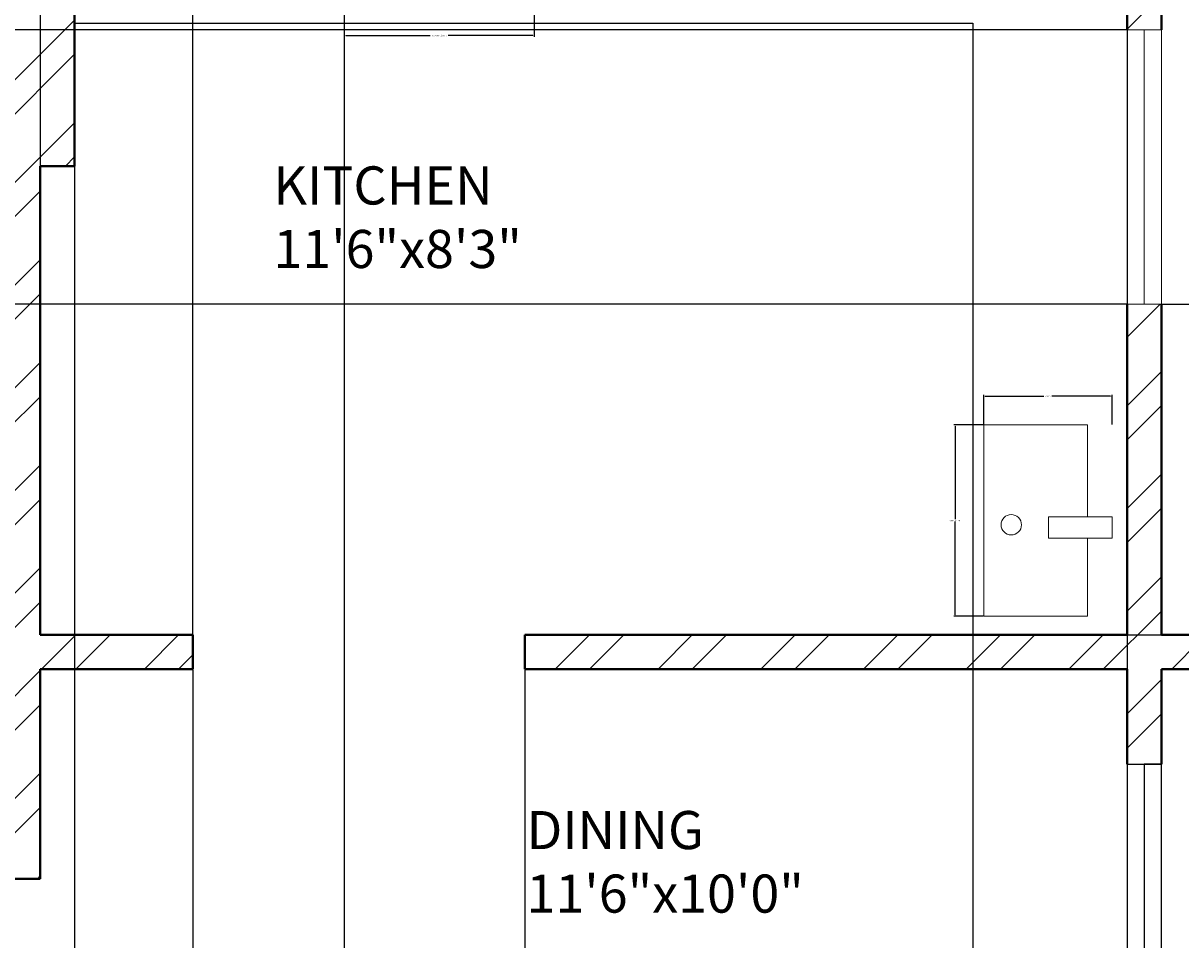
# Model space of a CAD drawing. Units: inches. Extents: x 1601 to 2297, y 1496 to 2631.
# Tile 27 of 57: x 2033 to 2185, y 1946 to 2067. Entities that reach past the tile are written whole.
import ezdxf

# ---------------------------------------------------------------- set-up
doc = ezdxf.new("R2010")
doc.units = ezdxf.units.IN
for name, color, linetype, lineweight in [('A-ANNO-DIMS', 2, 'Continuous', 18), ('A-AREA-IDEN', 7, 'Continuous', 18), ('A-DOOR', 21, 'Continuous', 25), ('A-FLOR-CASE', 8, 'Continuous', 25), ('A-FLOR-FIXT', 9, 'Continuous', 20), ('A-GLAZ', 161, 'Continuous', 20), ('A-WALL', 7, 'Continuous', 40), ('A-WALL-PATT', 215, 'Continuous', 13)]:
    doc.layers.add(name, color=color, linetype=linetype, lineweight=lineweight)
doc.styles.get("Standard").update_dxf_attribs({"font": 'arial.ttf'})
doc.dimstyles.get("Standard").update_dxf_attribs({"dimtxt": 0.18, "dimasz": 0.18, "dimexe": 0.18, "dimexo": 0.0625, "dimgap": 0.09, "dimtad": 0, "dimtih": 1, "dimtoh": 1, "dimdec": 4, "dimzin": 0, "dimdsep": 46, "dimtxsty": 'Standard', "dimcen": 0.09, "dimadec": 0, "dimazin": 0, "dimtfac": 1, "dimtdec": 4, "dimtofl": 0, "dimtmove": 0, "dimatfit": 3, "dimfxl": 1, "dimtolj": 1, "dimtzin": 0, "dimarcsym": 0})

# ---------------------------------------------------------------- blocks, each defined once
blk = doc.blocks.new('SINK-KITCHEN')
blk.add_lwpolyline([(13.62, 10.25), (13.62, 0), (0, 0), (0, 25.08), (13.62, 25.08), (13.62, 13.01)])
blk.add_lwpolyline([(8.47, 13.01), (16.82, 13.01), (16.82, 10.25), (8.47, 10.25)], close=True)
blk.add_circle((3.61, 11.99), 1.34)
blk = doc.blocks.new('*D18')
at = {"layer": 'A-ANNO-DIMS', "color": 0, "lineweight": -2, "transparency": 16777216}
for p, q in [((2075.4, 2068.63), (2075.4, 2064.77)), ((2100.29, 2068.63), (2100.29, 2064.77)), ((2075.58, 2064.95), (2086.65, 2064.95)), ((2100.11, 2064.95), (2089.03, 2064.95))]:
    blk.add_line(p, q, dxfattribs=at)
at = {"layer": 'A-ANNO-DIMS', "color": 0, "transparency": 16777216}
for points in [[(2075.58, 2064.98), (2075.58, 2064.92), (2075.4, 2064.95)], [(2100.11, 2064.98), (2100.11, 2064.92), (2100.29, 2064.95)]]:
    blk.add_solid(points, dxfattribs=at)
at = {"layer": 'Defpoints', "color": 0, "transparency": 16777216}
for p in [(2075.4, 2068.69), (2100.29, 2068.69), (2100.29, 2064.95)]:
    blk.add_point(p, dxfattribs=at)
at = {"layer": 'A-ANNO-DIMS', "color": 0, "transparency": 16777216, "insert": (2087.84, 2064.95), "char_height": 0.18, "attachment_point": 5}
blk.add_mtext('\\A1;COOKTOP 25 TYP.', dxfattribs=at)
blk = doc.blocks.new('*D20')
at = {"layer": 'A-ANNO-DIMS', "color": 0, "lineweight": -2, "transparency": 16777216}
for p, q in [((2159.18, 2013.87), (2155.3, 2013.87)), ((2155.48, 2013.69), (2155.48, 2001.51)), ((2155.48, 1988.97), (2155.48, 2001.14)), ((2159.18, 1988.79), (2155.3, 1988.79))]:
    blk.add_line(p, q, dxfattribs=at)
at = {"layer": 'A-ANNO-DIMS', "color": 0, "transparency": 16777216}
for points in [[(2155.45, 2013.69), (2155.51, 2013.69), (2155.48, 2013.87)], [(2155.45, 1988.97), (2155.51, 1988.97), (2155.48, 1988.79)]]:
    blk.add_solid(points, dxfattribs=at)
at = {"layer": 'Defpoints', "color": 0, "transparency": 16777216}
for p in [(2155.48, 2013.87), (2159.24, 2013.87), (2159.24, 1988.79)]:
    blk.add_point(p, dxfattribs=at)
at = {"layer": 'A-ANNO-DIMS', "color": 0, "transparency": 16777216, "insert": (2155.48, 2001.33), "char_height": 0.18, "attachment_point": 5}
blk.add_mtext('\\A1;SINK 25 TYP.', dxfattribs=at)
blk = doc.blocks.new('*D21')
at = {"layer": 'A-ANNO-DIMS', "color": 0, "lineweight": -2, "transparency": 16777216}
for p, q in [((2159.24, 2013.93), (2159.24, 2017.81)), ((2159.42, 2017.63), (2167.13, 2017.63)), ((2175.88, 2017.63), (2168.17, 2017.63)), ((2176.06, 2013.93), (2176.06, 2017.81))]:
    blk.add_line(p, q, dxfattribs=at)
at = {"layer": 'A-ANNO-DIMS', "color": 0, "transparency": 16777216}
for points in [[(2159.42, 2017.66), (2159.42, 2017.6), (2159.24, 2017.63)], [(2175.88, 2017.66), (2175.88, 2017.6), (2176.06, 2017.63)]]:
    blk.add_solid(points, dxfattribs=at)
at = {"layer": 'Defpoints', "color": 0, "transparency": 16777216}
for p in [(2176.06, 2017.63), (2159.24, 2013.87), (2176.06, 2013.87)]:
    blk.add_point(p, dxfattribs=at)
at = {"layer": 'A-ANNO-DIMS', "color": 0, "transparency": 16777216, "insert": (2167.65, 2017.63), "char_height": 0.18, "attachment_point": 5}
blk.add_mtext('\\A1;17 TYP.', dxfattribs=at)
blk = doc.blocks.new('*D38')
at = {"layer": 'A-ANNO-DIMS', "color": 0, "lineweight": -2, "transparency": 16777216}
for p, q in [((2178.04, 2085.26), (2178.04, 1513.75)), ((2157.8, 2066.51), (2157.8, 1513.75)), ((2157.98, 1513.93), (2167.52, 1513.93)), ((2177.86, 1513.93), (2168.31, 1513.93))]:
    blk.add_line(p, q, dxfattribs=at)
at = {"layer": 'A-ANNO-DIMS', "color": 0, "transparency": 16777216}
for points in [[(2157.98, 1513.96), (2157.98, 1513.9), (2157.8, 1513.93)], [(2177.86, 1513.96), (2177.86, 1513.9), (2178.04, 1513.93)]]:
    blk.add_solid(points, dxfattribs=at)
at = {"layer": 'Defpoints', "color": 0, "transparency": 16777216}
for p in [(2178.04, 2085.33), (2157.8, 2066.58), (2178.04, 1513.93)]:
    blk.add_point(p, dxfattribs=at)
at = {"layer": 'A-ANNO-DIMS', "color": 0, "transparency": 16777216, "insert": (2167.92, 1513.93), "char_height": 0.18, "attachment_point": 5}
blk.add_mtext('\\A1;20.24', dxfattribs=at)
blk = doc.blocks.new('*D39')
at = {"layer": 'A-ANNO-DIMS', "color": 0, "lineweight": -2, "transparency": 16777216}
for p, q in [((2055.55, 1981.76), (2055.55, 1513.75)), ((2099.05, 1981.76), (2099.05, 1513.75)), ((2055.73, 1513.93), (2076.97, 1513.93)), ((2098.87, 1513.93), (2077.63, 1513.93))]:
    blk.add_line(p, q, dxfattribs=at)
at = {"layer": 'A-ANNO-DIMS', "color": 0, "transparency": 16777216}
for points in [[(2055.73, 1513.96), (2055.73, 1513.9), (2055.55, 1513.93)], [(2098.87, 1513.96), (2098.87, 1513.9), (2099.05, 1513.93)]]:
    blk.add_solid(points, dxfattribs=at)
at = {"layer": 'Defpoints', "color": 0, "transparency": 16777216}
for p in [(2055.55, 1981.83), (2099.05, 1981.83), (2099.05, 1513.93)]:
    blk.add_point(p, dxfattribs=at)
at = {"layer": 'A-ANNO-DIMS', "color": 0, "transparency": 16777216, "insert": (2077.3, 1513.93), "char_height": 0.18, "attachment_point": 5}
blk.add_mtext('\\A1;43.5', dxfattribs=at)
blk = doc.blocks.new('*D40')
at = {"layer": 'A-ANNO-DIMS', "color": 0, "lineweight": -2, "transparency": 16777216}
for p, q in [((2035.54, 1986.39), (2035.54, 2581.06)), ((2035.72, 2580.88), (2045.08, 2580.88)), ((2055.37, 2580.88), (2046.01, 2580.88)), ((2055.55, 1986.39), (2055.55, 2581.06))]:
    blk.add_line(p, q, dxfattribs=at)
at = {"layer": 'A-ANNO-DIMS', "color": 0, "transparency": 16777216}
for points in [[(2035.72, 2580.91), (2035.72, 2580.85), (2035.54, 2580.88)], [(2055.37, 2580.91), (2055.37, 2580.85), (2055.55, 2580.88)]]:
    blk.add_solid(points, dxfattribs=at)
at = {"layer": 'Defpoints', "color": 0, "transparency": 16777216}
for p in [(2055.55, 2580.88), (2035.54, 1986.33), (2055.55, 1986.33)]:
    blk.add_point(p, dxfattribs=at)
at = {"layer": 'A-ANNO-DIMS', "color": 0, "transparency": 16777216, "insert": (2045.54, 2580.88), "char_height": 0.18, "attachment_point": 5}
blk.add_mtext('\\A1;20.014', dxfattribs=at)
blk = doc.blocks.new('*D41')
at = {"layer": 'A-ANNO-DIMS', "color": 0, "lineweight": -2, "transparency": 16777216}
for p, q in [((2075.4, 2070.14), (2075.4, 1513.75)), ((2040.04, 2066.51), (2040.04, 1513.75)), ((2040.22, 1513.93), (2057.32, 1513.93)), ((2075.22, 1513.93), (2058.11, 1513.93))]:
    blk.add_line(p, q, dxfattribs=at)
at = {"layer": 'A-ANNO-DIMS', "color": 0, "transparency": 16777216}
for points in [[(2040.22, 1513.96), (2040.22, 1513.9), (2040.04, 1513.93)], [(2075.22, 1513.96), (2075.22, 1513.9), (2075.4, 1513.93)]]:
    blk.add_solid(points, dxfattribs=at)
at = {"layer": 'Defpoints', "color": 0, "transparency": 16777216}
for p in [(2075.4, 2070.2), (2040.04, 2066.58), (2075.4, 1513.93)]:
    blk.add_point(p, dxfattribs=at)
at = {"layer": 'A-ANNO-DIMS', "color": 0, "transparency": 16777216, "insert": (2057.72, 1513.93), "char_height": 0.18, "attachment_point": 5}
blk.add_mtext('\\A1;35.36', dxfattribs=at)
blk = doc.blocks.new('*D42')
at = {"layer": 'A-ANNO-DIMS', "color": 0, "lineweight": -2, "transparency": 16777216}
for p, q in [((2177.97, 2065.7), (1637.31, 2065.7)), ((1637.49, 2065.52), (1637.49, 2047.88)), ((1637.49, 2029.88), (1637.49, 2047.51)), ((2177.97, 2029.7), (1637.31, 2029.7))]:
    blk.add_line(p, q, dxfattribs=at)
at = {"layer": 'A-ANNO-DIMS', "color": 0, "transparency": 16777216}
for points in [[(1637.46, 2065.52), (1637.52, 2065.52), (1637.49, 2065.7)], [(1637.46, 2029.88), (1637.52, 2029.88), (1637.49, 2029.7)]]:
    blk.add_solid(points, dxfattribs=at)
at = {"layer": 'Defpoints', "color": 0, "transparency": 16777216}
for p in [(1637.49, 2065.7), (2178.04, 2065.7), (2178.04, 2029.7)]:
    blk.add_point(p, dxfattribs=at)
at = {"layer": 'A-ANNO-DIMS', "color": 0, "transparency": 16777216, "insert": (1637.49, 2047.7), "char_height": 0.18, "attachment_point": 5}
blk.add_mtext('\\A1;36', dxfattribs=at)
blk = doc.blocks.new('*D43')
at = {"layer": 'A-ANNO-DIMS', "color": 0, "lineweight": -2, "transparency": 16777216}
for p, q in [((2182.6, 2029.7), (2279.27, 2029.7)), ((2279.09, 2029.52), (2279.09, 2008.19)), ((2279.09, 1986.51), (2279.09, 2007.83)), ((2178.1, 1986.33), (2279.27, 1986.33))]:
    blk.add_line(p, q, dxfattribs=at)
at = {"layer": 'A-ANNO-DIMS', "color": 0, "transparency": 16777216}
for points in [[(2279.06, 2029.52), (2279.12, 2029.52), (2279.09, 2029.7)], [(2279.06, 1986.51), (2279.12, 1986.51), (2279.09, 1986.33)]]:
    blk.add_solid(points, dxfattribs=at)
at = {"layer": 'Defpoints', "color": 0, "transparency": 16777216}
for p in [(2182.54, 2029.7), (2178.04, 1986.33), (2279.09, 1986.33)]:
    blk.add_point(p, dxfattribs=at)
at = {"layer": 'A-ANNO-DIMS', "color": 0, "transparency": 16777216, "insert": (2279.09, 2008.01), "char_height": 0.18, "attachment_point": 5}
blk.add_mtext('\\A1;43.37', dxfattribs=at)

msp = doc.modelspace()

# ---------------------------------------------------------------- hatches: boundary and pattern name
at = {"layer": 'A-WALL-PATT'}
h = msp.add_hatch(dxfattribs=at)
h.set_pattern_fill('ANSI32', color=256)
h.paths.add_polyline_path([(1842.0336, 2528.0767), (1842.0336, 2532.3254), (1686.0373, 2532.3254), (1686.0373, 2492.9493), (1695.0373, 2492.9493), (1695.0373, 2523.3254), (1827.0373, 2523.3254), (1827.0373, 2416.8254), (1834.6225, 2416.8254), (1834.6225, 2419.0754), (1834.6225, 2421.3254), (1831.5373, 2421.3254), (1831.5373, 2523.3254), (1842.0336, 2523.3254)])
h.paths.add_polyline_path([(1695.0373, 2432.9493), (1686.0373, 2432.9493), (1686.0373, 2325.989), (1695.0373, 2325.989), (1695.0373, 2347.8254), (1827.0373, 2347.8254), (1827.0373, 2287.8254), (1823.2991, 2287.8254), (1823.2991, 2283.3254), (1847.9422, 2283.3254), (1847.9422, 2285.5754), (1847.9422, 2287.8254), (1831.5373, 2287.8254), (1831.5373, 2347.8254), (1846.9946, 2347.8254), (1846.9946, 2350.0754), (1846.9946, 2352.3254), (1695.0373, 2352.3254)])
h.paths.add_polyline_path([(1807.1169, 1573.5395), (2055.0405, 1573.5395), (2055.0405, 1610.6322), (1807.1169, 1610.6322)], flags=9)
h.paths.add_polyline_path([(1841.1631, 1712.7967), (1870.3957, 1712.7967), (1870.3957, 1731.454), (1841.1631, 1731.454)], flags=9)
h.paths.add_polyline_path([(2144.3862, 1772.185), (2191.0233, 1772.185), (2191.0233, 1790.8423), (2144.3862, 1790.8423)], flags=9)
h.paths.add_polyline_path([(2143.0128, 1827.3312), (2177.9958, 1827.3312), (2177.9958, 1845.9886), (2143.0128, 1845.9886)], flags=9)
h.paths.add_polyline_path([(2041.2439, 1833.5691), (2070.8516, 1833.5691), (2070.8516, 1852.2264), (2041.2439, 1852.2264)], flags=9)
h.paths.add_polyline_path([(2097.2791, 1947.0598), (2134.2061, 1947.0598), (2134.2061, 1965.7171), (2097.2791, 1965.7171)], flags=9)
h.paths.add_polyline_path([(2214.995, 1904.3124), (2214.995, 1942.2899), (2196.3376, 1942.2899), (2196.3376, 1904.3124)], flags=9)
h.paths.add_polyline_path([(2186.6284, 2043.8031), (2219.7935, 2043.8031), (2219.7935, 2062.4605), (2186.6284, 2062.4605)], flags=9)
h.paths.add_polyline_path([(2064.0877, 2031.616), (2097.4949, 2031.616), (2097.4949, 2050.2734), (2064.0877, 2050.2734)], flags=9)
h.paths.add_polyline_path([(1973.1349, 1986.0688), (2008.4009, 1986.0688), (2008.4009, 2004.7261), (1973.1349, 2004.7261)], flags=9)
h.paths.add_polyline_path([(1976.3676, 2106.9635), (2005.7469, 2106.9635), (2005.7469, 2125.6209), (1976.3676, 2125.6209)], flags=9)
h.paths.add_polyline_path([(1991.7852, 2180.4863), (2027.0513, 2180.4863), (2027.0513, 2199.1437), (1991.7852, 2199.1437)], flags=9)
h.paths.add_polyline_path([(2106.1801, 2187.9359), (2152.2101, 2187.9359), (2152.2101, 2206.5932), (2106.1801, 2206.5932)], flags=9)
h.paths.add_polyline_path([(2148.6686, 2262.2542), (2182.318, 2262.2542), (2182.318, 2280.9115), (2148.6686, 2280.9115)], flags=9)
h.paths.add_polyline_path([(2041.6327, 2252.8147), (2071.2405, 2252.8147), (2071.2405, 2271.4721), (2041.6327, 2271.4721)], flags=9)
h.paths.add_polyline_path([(2063.9734, 2375.4265), (2100.9004, 2375.4265), (2100.9004, 2394.0839), (2063.9734, 2394.0839)], flags=9)
h.paths.add_polyline_path([(2216.4955, 2330.9748), (2216.4955, 2370.2654), (2197.8381, 2370.2654), (2197.8381, 2330.9748)], flags=9)
h.paths.add_polyline_path([(2179.1416, 2485.8687), (2212.3067, 2485.8687), (2212.3067, 2504.5261), (2179.1416, 2504.5261)], flags=9)
h.paths.add_polyline_path([(2078.7442, 2471.1516), (2112.1514, 2471.1516), (2112.1514, 2489.809), (2078.7442, 2489.809)], flags=9)
h.paths.add_polyline_path([(1915.9631, 2329.4668), (1952.8902, 2329.4668), (1952.8902, 2348.1241), (1915.9631, 2348.1241)], flags=9)
h.paths.add_polyline_path([(1904.3189, 2499.6709), (1940.4512, 2499.6709), (1940.4512, 2518.3282), (1904.3189, 2518.3282)], flags=9)
h.paths.add_polyline_path([(1892.3665, 2100.4595), (1925.6374, 2100.4595), (1925.6374, 2119.1169), (1892.3665, 2119.1169)], flags=9)
h.paths.add_polyline_path([(1909.2984, 1805.9631), (1946.2254, 1805.9631), (1946.2254, 1824.6205), (1909.2984, 1824.6205)], flags=9)
h.paths.add_polyline_path([(1934.6056, 1658.616), (1970.738, 1658.616), (1970.738, 1677.2733), (1934.6056, 1677.2733)], flags=9)
h.paths.add_polyline_path([(1711.2052, 1789.8902), (1750.0456, 1789.8902), (1750.0456, 1808.5476), (1711.2052, 1808.5476)], flags=9)
h.paths.add_polyline_path([(1742.7874, 1854.6743), (1771.9449, 1854.6743), (1771.9449, 1873.3317), (1742.7874, 1873.3317)], flags=9)
h.paths.add_polyline_path([(1807.3592, 1997.7912), (1850.1116, 1997.7912), (1850.1116, 2016.4486), (1807.3592, 2016.4486)], flags=9)
h.paths.add_polyline_path([(1717.4579, 2237.7844), (1760.2103, 2237.7844), (1760.2103, 2256.4417), (1717.4579, 2256.4417)], flags=9)
h.paths.add_polyline_path([(1780.9285, 2324.0623), (1810.086, 2324.0623), (1810.086, 2342.7197), (1780.9285, 2342.7197)], flags=25)
h.paths.add_polyline_path([(1837.696, 2449.2024), (1866.9286, 2449.2024), (1866.9286, 2467.8598), (1837.696, 2467.8598)], flags=9)
h.paths.add_polyline_path([(1712.7752, 2484.9404), (1751.6156, 2484.9404), (1751.6156, 2503.5977), (1712.7752, 2503.5977)], flags=25)
h = msp.add_hatch(dxfattribs=at)
h.set_pattern_fill('ANSI32', color=256)
h.paths.add_polyline_path([(1973.9371, 2211.3254), (1893.0373, 2211.3254), (1893.0373, 2287.8254), (1884.6167, 2287.8254), (1884.6167, 2285.5754), (1884.6167, 2283.3254), (1888.5373, 2283.3254), (1888.5373, 2145.3254), (1695.0373, 2145.3254), (1695.0373, 2173.8724), (1690.5373, 2173.8724), (1686.0373, 2173.8724), (1686.0373, 2136.3254), (1722.5687, 2136.3254), (1722.5687, 2117.4352), (1731.5687, 2117.4352), (1731.5687, 2136.3254), (1893.0373, 2136.3254), (1893.0373, 2202.3254), (1959.0373, 2202.3254), (1959.0373, 2182.1303), (1968.0373, 2182.1303), (1968.0373, 2202.3254), (1973.9371, 2202.3254)])
h.paths.add_polyline_path([(2094.0373, 2274.6364), (2096.4294, 2274.6364), (2096.4294, 2276.8864), (2096.4294, 2279.1364), (2094.0373, 2279.1364), (2094.0373, 2290.8254), (2094.0373, 2295.3254), (2089.5373, 2295.3254), (2089.5373, 2230.8254), (2035.5373, 2230.8254), (2035.5373, 2299.8254), (2031.0373, 2299.8254), (2031.0373, 2211.3254), (2023.0065, 2211.3254), (2023.0065, 2202.3254), (2031.0373, 2202.3254), (2031.0373, 2140.8254), (1968.0373, 2140.8254), (1968.0373, 2145.9106), (1963.5373, 2145.9106), (1959.0373, 2145.9106), (1959.0373, 2116.839), (1963.5373, 2116.839), (1968.0373, 2116.839), (1968.0373, 2131.8254), (2031.0373, 2131.8254), (2031.0373, 2094.3254), (2031.0373, 2085.3254), (2031.0373, 2056.8254), (1968.0373, 2056.8254), (1968.0373, 2070.4947), (1963.5373, 2070.4947), (1959.0373, 2070.4947), (1959.0373, 2040.3029), (1968.0373, 2040.3029), (1968.0373, 2047.8254), (2031.0373, 2047.8254), (2031.0373, 1983.3254), (2031.0373, 1978.8254), (2021.1979, 1978.8254), (2021.1979, 1974.3254), (2031.0373, 1974.3254), (2031.0373, 1954.3528), (2035.5373, 1954.3528), (2035.5373, 1974.3254), (2035.5373, 1981.8254), (2055.5513, 1981.8254), (2055.5513, 1986.3254), (2035.5373, 1986.3254), (2035.5373, 2047.8254), (2040.0373, 2047.8254), (2040.0373, 2085.3254), (2040.0373, 2094.3254), (2040.0373, 2140.8254), (2035.5373, 2140.8254), (2035.5373, 2226.3254), (2089.5373, 2226.3254), (2094.0373, 2226.3254)])
h.paths.add_polyline_path([(2226.0373, 2230.8254), (2134.5373, 2230.8254), (2134.5373, 2233.5437), (2130.0373, 2233.5437), (2130.0373, 2226.3254), (2134.5373, 2226.3254), (2226.0373, 2226.3254)])
h.paths.add_polyline_path([(1807.1169, 1573.5395), (2055.0405, 1573.5395), (2055.0405, 1610.6322), (1807.1169, 1610.6322)], flags=9)
h.paths.add_polyline_path([(1841.1631, 1712.7967), (1870.3957, 1712.7967), (1870.3957, 1731.454), (1841.1631, 1731.454)], flags=9)
h.paths.add_polyline_path([(2144.3862, 1772.185), (2191.0233, 1772.185), (2191.0233, 1790.8423), (2144.3862, 1790.8423)], flags=9)
h.paths.add_polyline_path([(2143.0128, 1827.3312), (2177.9958, 1827.3312), (2177.9958, 1845.9886), (2143.0128, 1845.9886)], flags=9)
h.paths.add_polyline_path([(2041.2439, 1833.5691), (2070.8516, 1833.5691), (2070.8516, 1852.2264), (2041.2439, 1852.2264)], flags=9)
h.paths.add_polyline_path([(2097.2791, 1947.0598), (2134.2061, 1947.0598), (2134.2061, 1965.7171), (2097.2791, 1965.7171)], flags=9)
h.paths.add_polyline_path([(2214.995, 1904.3124), (2214.995, 1942.2899), (2196.3376, 1942.2899), (2196.3376, 1904.3124)], flags=9)
h.paths.add_polyline_path([(2186.6284, 2043.8031), (2219.7935, 2043.8031), (2219.7935, 2062.4605), (2186.6284, 2062.4605)], flags=9)
h.paths.add_polyline_path([(2064.0877, 2031.616), (2097.4949, 2031.616), (2097.4949, 2050.2734), (2064.0877, 2050.2734)], flags=9)
h.paths.add_polyline_path([(1973.1349, 1986.0688), (2008.4009, 1986.0688), (2008.4009, 2004.7261), (1973.1349, 2004.7261)], flags=25)
h.paths.add_polyline_path([(1976.3676, 2106.9635), (2005.7469, 2106.9635), (2005.7469, 2125.6209), (1976.3676, 2125.6209)], flags=25)
h.paths.add_polyline_path([(1991.7852, 2180.4863), (2027.0513, 2180.4863), (2027.0513, 2199.1437), (1991.7852, 2199.1437)], flags=25)
h.paths.add_polyline_path([(2106.1801, 2187.9359), (2152.2101, 2187.9359), (2152.2101, 2206.5932), (2106.1801, 2206.5932)], flags=9)
h.paths.add_polyline_path([(2148.6686, 2262.2542), (2182.318, 2262.2542), (2182.318, 2280.9115), (2148.6686, 2280.9115)], flags=9)
h.paths.add_polyline_path([(2041.6327, 2252.8147), (2071.2405, 2252.8147), (2071.2405, 2271.4721), (2041.6327, 2271.4721)], flags=25)
h.paths.add_polyline_path([(2063.9734, 2375.4265), (2100.9004, 2375.4265), (2100.9004, 2394.0839), (2063.9734, 2394.0839)], flags=9)
h.paths.add_polyline_path([(2216.4955, 2330.9748), (2216.4955, 2370.2654), (2197.8381, 2370.2654), (2197.8381, 2330.9748)], flags=9)
h.paths.add_polyline_path([(2179.1416, 2485.8687), (2212.3067, 2485.8687), (2212.3067, 2504.5261), (2179.1416, 2504.5261)], flags=9)
h.paths.add_polyline_path([(2078.7442, 2471.1516), (2112.1514, 2471.1516), (2112.1514, 2489.809), (2078.7442, 2489.809)], flags=9)
h.paths.add_polyline_path([(1915.9631, 2329.4668), (1952.8902, 2329.4668), (1952.8902, 2348.1241), (1915.9631, 2348.1241)], flags=9)
h.paths.add_polyline_path([(1904.3189, 2499.6709), (1940.4512, 2499.6709), (1940.4512, 2518.3282), (1904.3189, 2518.3282)], flags=9)
h.paths.add_polyline_path([(1892.3665, 2100.4595), (1925.6374, 2100.4595), (1925.6374, 2119.1169), (1892.3665, 2119.1169)], flags=9)
h.paths.add_polyline_path([(1909.2984, 1805.9631), (1946.2254, 1805.9631), (1946.2254, 1824.6205), (1909.2984, 1824.6205)], flags=9)
h.paths.add_polyline_path([(1934.6056, 1658.616), (1970.738, 1658.616), (1970.738, 1677.2733), (1934.6056, 1677.2733)], flags=9)
h.paths.add_polyline_path([(1711.2052, 1789.8902), (1750.0456, 1789.8902), (1750.0456, 1808.5476), (1711.2052, 1808.5476)], flags=9)
h.paths.add_polyline_path([(1742.7874, 1854.6743), (1771.9449, 1854.6743), (1771.9449, 1873.3317), (1742.7874, 1873.3317)], flags=9)
h.paths.add_polyline_path([(1807.3592, 1997.7912), (1850.1116, 1997.7912), (1850.1116, 2016.4486), (1807.3592, 2016.4486)], flags=9)
h.paths.add_polyline_path([(1717.4579, 2237.7844), (1760.2103, 2237.7844), (1760.2103, 2256.4417), (1717.4579, 2256.4417)], flags=25)
h.paths.add_polyline_path([(1780.9285, 2324.0623), (1810.086, 2324.0623), (1810.086, 2342.7197), (1780.9285, 2342.7197)], flags=9)
h.paths.add_polyline_path([(1837.696, 2449.2024), (1866.9286, 2449.2024), (1866.9286, 2467.8598), (1837.696, 2467.8598)], flags=9)
h.paths.add_polyline_path([(1712.7752, 2484.9404), (1751.6156, 2484.9404), (1751.6156, 2503.5977), (1712.7752, 2503.5977)], flags=9)
h = msp.add_hatch(dxfattribs=at)
h.set_pattern_fill('ANSI32', color=256)
h.paths.add_polyline_path([(2230.5373, 1861.8254), (2182.5373, 1861.8254), (2182.5373, 1885.3637), (2178.0373, 1885.3637), (2178.0373, 1861.8254), (2166.0373, 1861.8254), (2134.5373, 1861.8254), (2130.0373, 1861.8254), (2130.0373, 1841.4682), (2126.8833, 1841.4682), (2126.8833, 1836.9682), (2130.0373, 1836.9682), (2130.0373, 1822.7302), (2134.5373, 1822.7302), (2134.5373, 1857.3254), (2166.0373, 1857.3254), (2226.0373, 1857.3254), (2226.0373, 1846.1155), (2230.5373, 1846.1155)])
h.paths.add_polyline_path([(2226.0373, 1797.3254), (2134.5373, 1797.3254), (2134.5373, 1800.6636), (2132.2873, 1800.6636), (2130.0373, 1800.6636), (2130.0373, 1797.3254), (2130.0373, 1792.8254), (2167.7264, 1792.8254), (2226.0373, 1792.8254)])
h.paths.add_polyline_path([(2230.5373, 1822.1155), (2226.0373, 1822.1155), (2226.0373, 1760.8563), (2230.5373, 1760.8563)])
h.paths.add_polyline_path([(2230.5373, 1700.8563), (2226.0373, 1700.8563), (2226.0373, 1644.3254), (2140.2517, 1644.3254), (2140.2517, 1635.3254), (2230.5373, 1635.3254)])
h.paths.add_polyline_path([(2080.2517, 1639.8254), (2080.2517, 1644.3254), (2035.5373, 1644.3254), (2035.5373, 1792.8254), (2094.0373, 1792.8254), (2094.0373, 1797.3254), (2094.0373, 1836.9682), (2097.1057, 1836.9682), (2097.1057, 1839.2182), (2097.1057, 1841.4682), (2094.0373, 1841.4682), (2094.0373, 1862.2276), (2089.5373, 1862.2276), (2089.5373, 1797.3254), (2035.5373, 1797.3254), (2035.5373, 1857.3254), (2035.5373, 1885.0916), (2031.0373, 1885.0916), (2031.0373, 1710.3254), (2012.329, 1710.3254), (2012.329, 1701.3254), (2031.0373, 1701.3254), (2031.0373, 1644.3254), (2031.0373, 1635.3254), (2080.2517, 1635.3254)])
h.paths.add_polyline_path([(1836.0373, 1653.2033), (1842.6171, 1653.2033), (1842.6171, 1657.7033), (1842.6171, 1662.2033), (1831.5373, 1662.2033), (1831.5373, 1764.2033), (1835.3881, 1764.2033), (1835.3881, 1766.4533), (1835.3881, 1768.7033), (1831.5373, 1768.7033), (1827.0373, 1768.7033), (1827.0373, 1662.2033), (1827.0373, 1635.3254), (1836.0373, 1635.3254)])
h.paths.add_polyline_path([(1893.0373, 1701.3254), (1907.193, 1701.3254), (1907.193, 1705.8254), (1907.193, 1710.3254), (1893.0373, 1710.3254), (1893.0373, 1819.8254), (1882.6444, 1819.8254), (1882.6444, 1817.5754), (1882.6444, 1815.3254), (1888.5373, 1815.3254), (1888.5373, 1662.2033), (1884.0373, 1662.2033), (1866.6171, 1662.2033), (1866.6171, 1653.2033), (1882.391, 1653.2033), (1884.0373, 1653.2033), (1884.0373, 1635.3254), (1893.0373, 1635.3254)])
h.paths.add_polyline_path([(1739.3335, 1639.8254), (1739.3335, 1644.3254), (1695.0373, 1644.3254), (1695.0373, 1702.0135), (1690.5373, 1702.0135), (1686.0373, 1702.0135), (1686.0373, 1635.3254), (1739.3335, 1635.3254)])
h.paths.add_polyline_path([(1827.0373, 1644.3254), (1799.3335, 1644.3254), (1799.3335, 1635.3254), (1827.0373, 1635.3254)])
h.paths.add_polyline_path([(1695.0373, 1815.3254), (1849.2759, 1815.3254), (1849.2759, 1819.8254), (1807.5373, 1819.8254), (1807.5373, 1879.8254), (1851.1533, 1879.8254), (1851.1533, 1882.0754), (1851.1533, 1884.3254), (1799.3405, 1884.3254), (1799.3405, 1882.0754), (1799.3405, 1879.8254), (1803.0373, 1879.8254), (1803.0373, 1819.8254), (1695.0373, 1819.8254), (1695.0373, 1835.0458), (1690.5373, 1835.0458), (1686.0373, 1835.0458), (1686.0373, 1766.1753), (1695.0373, 1766.1753)])
h.paths.add_polyline_path([(1775.8157, 1884.3254), (1695.0373, 1884.3254), (1695.0373, 1912.9526), (1690.5373, 1912.9526), (1686.0373, 1912.9526), (1686.0373, 1859.0458), (1695.0373, 1859.0458), (1695.0373, 1879.8254), (1775.8157, 1879.8254)])
h.paths.add_polyline_path([(1893.0373, 2031.3254), (1731.5687, 2031.3254), (1731.5687, 2057.4352), (1722.5687, 2057.4352), (1722.5687, 2031.3254), (1686.0373, 2031.3254), (1686.0373, 1972.9526), (1695.0373, 1972.9526), (1695.0373, 2022.3254), (1888.5373, 2022.3254), (1888.5373, 1884.3254), (1883.4996, 1884.3254), (1883.4996, 1879.8254), (1893.0373, 1879.8254), (1893.0373, 1974.3254), (1976.6199, 1974.3254), (1976.6199, 1978.8254), (1968.0373, 1978.8254), (1968.0373, 1983.3254), (1968.0373, 2008.4756), (1963.5373, 2008.4756), (1959.0373, 2008.4756), (1959.0373, 1983.3254), (1893.0373, 1983.3254)])
h.paths.add_polyline_path([(2230.5373, 2140.4745), (2226.0373, 2140.4745), (2226.0373, 2094.3254), (2040.0373, 2094.3254), (2040.0373, 2085.3254), (2178.0373, 2085.3254), (2178.0373, 2065.6965), (2182.5373, 2065.6965), (2182.5373, 2085.3254), (2226.0373, 2085.3254), (2226.0373, 1986.3254), (2211.2679, 1986.3254), (2211.2679, 1981.8254), (2230.5373, 1981.8254)])
h.paths.add_polyline_path([(2187.6292, 1986.3254), (2182.5373, 1986.3254), (2182.5373, 2029.6965), (2178.0373, 2029.6965), (2178.0373, 1986.3254), (2099.05, 1986.3254), (2099.05, 1981.8254), (2178.0373, 1981.8254), (2178.0373, 1969.3637), (2182.5373, 1969.3637), (2182.5373, 1981.8254), (2187.6292, 1981.8254), (2187.6292, 1984.0754)])
h.paths.add_polyline_path([(1807.1169, 1573.5395), (2055.0405, 1573.5395), (2055.0405, 1610.6322), (1807.1169, 1610.6322)], flags=9)
h.paths.add_polyline_path([(1841.1631, 1712.7967), (1870.3957, 1712.7967), (1870.3957, 1731.454), (1841.1631, 1731.454)], flags=9)
h.paths.add_polyline_path([(2144.3862, 1772.185), (2191.0233, 1772.185), (2191.0233, 1790.8423), (2144.3862, 1790.8423)], flags=9)
h.paths.add_polyline_path([(2143.0128, 1827.3312), (2177.9958, 1827.3312), (2177.9958, 1845.9886), (2143.0128, 1845.9886)], flags=25)
h.paths.add_polyline_path([(2041.2439, 1833.5691), (2070.8516, 1833.5691), (2070.8516, 1852.2264), (2041.2439, 1852.2264)], flags=25)
h.paths.add_polyline_path([(2097.2791, 1947.0598), (2134.2061, 1947.0598), (2134.2061, 1965.7171), (2097.2791, 1965.7171)], flags=9)
h.paths.add_polyline_path([(2214.995, 1904.3124), (2214.995, 1942.2899), (2196.3376, 1942.2899), (2196.3376, 1904.3124)], flags=9)
h.paths.add_polyline_path([(2186.6284, 2043.8031), (2219.7935, 2043.8031), (2219.7935, 2062.4605), (2186.6284, 2062.4605)], flags=25)
h.paths.add_polyline_path([(2064.0877, 2031.616), (2097.4949, 2031.616), (2097.4949, 2050.2734), (2064.0877, 2050.2734)], flags=25)
h.paths.add_polyline_path([(1973.1349, 1986.0688), (2008.4009, 1986.0688), (2008.4009, 2004.7261), (1973.1349, 2004.7261)], flags=9)
h.paths.add_polyline_path([(1976.3676, 2106.9635), (2005.7469, 2106.9635), (2005.7469, 2125.6209), (1976.3676, 2125.6209)], flags=9)
h.paths.add_polyline_path([(1991.7852, 2180.4863), (2027.0513, 2180.4863), (2027.0513, 2199.1437), (1991.7852, 2199.1437)], flags=9)
h.paths.add_polyline_path([(2106.1801, 2187.9359), (2152.2101, 2187.9359), (2152.2101, 2206.5932), (2106.1801, 2206.5932)], flags=9)
h.paths.add_polyline_path([(2148.6686, 2262.2542), (2182.318, 2262.2542), (2182.318, 2280.9115), (2148.6686, 2280.9115)], flags=9)
h.paths.add_polyline_path([(2041.6327, 2252.8147), (2071.2405, 2252.8147), (2071.2405, 2271.4721), (2041.6327, 2271.4721)], flags=9)
h.paths.add_polyline_path([(2063.9734, 2375.4265), (2100.9004, 2375.4265), (2100.9004, 2394.0839), (2063.9734, 2394.0839)], flags=9)
h.paths.add_polyline_path([(2216.4955, 2330.9748), (2216.4955, 2370.2654), (2197.8381, 2370.2654), (2197.8381, 2330.9748)], flags=9)
h.paths.add_polyline_path([(2179.1416, 2485.8687), (2212.3067, 2485.8687), (2212.3067, 2504.5261), (2179.1416, 2504.5261)], flags=9)
h.paths.add_polyline_path([(2078.7442, 2471.1516), (2112.1514, 2471.1516), (2112.1514, 2489.809), (2078.7442, 2489.809)], flags=9)
h.paths.add_polyline_path([(1915.9631, 2329.4668), (1952.8902, 2329.4668), (1952.8902, 2348.1241), (1915.9631, 2348.1241)], flags=9)
h.paths.add_polyline_path([(1904.3189, 2499.6709), (1940.4512, 2499.6709), (1940.4512, 2518.3282), (1904.3189, 2518.3282)], flags=9)
h.paths.add_polyline_path([(1892.3665, 2100.4595), (1925.6374, 2100.4595), (1925.6374, 2119.1169), (1892.3665, 2119.1169)], flags=9)
h.paths.add_polyline_path([(1909.2984, 1805.9631), (1946.2254, 1805.9631), (1946.2254, 1824.6205), (1909.2984, 1824.6205)], flags=9)
h.paths.add_polyline_path([(1934.6056, 1658.616), (1970.738, 1658.616), (1970.738, 1677.2733), (1934.6056, 1677.2733)], flags=9)
h.paths.add_polyline_path([(1711.2052, 1789.8902), (1750.0456, 1789.8902), (1750.0456, 1808.5476), (1711.2052, 1808.5476)], flags=25)
h.paths.add_polyline_path([(1742.7874, 1854.6743), (1771.9449, 1854.6743), (1771.9449, 1873.3317), (1742.7874, 1873.3317)], flags=25)
h.paths.add_polyline_path([(1807.3592, 1997.7912), (1850.1116, 1997.7912), (1850.1116, 2016.4486), (1807.3592, 2016.4486)], flags=25)
h.paths.add_polyline_path([(1717.4579, 2237.7844), (1760.2103, 2237.7844), (1760.2103, 2256.4417), (1717.4579, 2256.4417)], flags=9)
h.paths.add_polyline_path([(1780.9285, 2324.0623), (1810.086, 2324.0623), (1810.086, 2342.7197), (1780.9285, 2342.7197)], flags=9)
h.paths.add_polyline_path([(1837.696, 2449.2024), (1866.9286, 2449.2024), (1866.9286, 2467.8598), (1837.696, 2467.8598)], flags=9)
h.paths.add_polyline_path([(1712.7752, 2484.9404), (1751.6156, 2484.9404), (1751.6156, 2503.5977), (1712.7752, 2503.5977)], flags=9)

# ---------------------------------------------------------------- linework, layer by layer
at = {"layer": 'A-DOOR'}
for p, q in [((2178.0373, 1969.3637), (2182.5373, 1969.3637)), ((2182.5373, 1969.3637), (2180.2873, 1969.3637)), ((2180.2873, 1969.3637), (2180.2873, 1885.3637)), ((2182.5373, 1916.3821), (2182.5373, 1969.3637))]:
    msp.add_line(p, q, dxfattribs=at)
at = {"layer": 'A-FLOR-CASE'}
for p, q in [((2040.0373, 2066.5754), (2157.799, 2066.5754)), ((2157.799, 2066.5754), (2157.799, 1986.3254))]:
    msp.add_line(p, q, dxfattribs=at)
at = {"layer": 'A-GLAZ'}
for p, q in [((2178.0373, 2065.6965), (2182.5373, 2065.6965)), ((2178.0373, 2065.6965), (2178.0373, 2029.6965)), ((2182.5373, 2065.6965), (2180.2873, 2065.6965)), ((2180.2873, 2065.6965), (2180.2873, 2029.6965)), ((2182.5373, 2065.6965), (2182.5373, 2029.6965)), ((2180.2873, 2029.6965), (2178.0373, 2029.6965)), ((2178.0373, 2029.6965), (2182.5373, 2029.6965))]:
    msp.add_line(p, q, dxfattribs=at)
at = {"layer": 'A-WALL'}
for p, q in [((2040.0373, 2085.3254), (2040.0373, 2047.8254)), ((2178.0373, 2085.3254), (2178.0373, 2065.6965)), ((2182.5373, 2065.6965), (2182.5373, 2085.3254)), ((2040.0373, 2047.8254), (2035.5373, 2047.8254)), ((2035.5373, 1986.3254), (2035.5373, 2047.8254)), ((2178.0373, 2029.6965), (2178.0373, 1986.3254)), ((2182.5373, 1986.3254), (2182.5373, 2029.6965)), ((2035.5373, 1986.3254), (2055.5513, 1986.3254)), ((2055.5513, 1986.3254), (2055.5513, 1981.8254)), ((2099.05, 1986.3254), (2099.05, 1981.8254)), ((2099.05, 1986.3254), (2178.0373, 1986.3254)), ((2182.5373, 1986.3254), (2189.6292, 1986.3254)), ((2035.5373, 1974.3254), (2035.5373, 1981.8254)), ((2035.5373, 1981.8254), (2055.5513, 1981.8254)), ((2099.05, 1981.8254), (2178.0373, 1981.8254)), ((2178.0373, 1969.3637), (2178.0373, 1981.8254)), ((2182.5373, 1981.8254), (2182.5373, 1969.3637)), ((2182.5373, 1981.8254), (2187.6292, 1981.8254)), ((2035.5373, 1974.3254), (2035.5373, 1954.3528)), ((2031.0373, 1954.3528), (2035.5373, 1954.3528))]:
    msp.add_line(p, q, dxfattribs=at)

# ---------------------------------------------------------------- block references
at = {"layer": 'A-FLOR-FIXT'}
msp.add_blockref('SINK-KITCHEN', (2159.239, 1988.787), dxfattribs=at)

# ---------------------------------------------------------------- texts
at = {"layer": 'A-AREA-IDEN', "char_height": 5, "attachment_point": 1}
for s, width, insert in [('KITCHEN\\P11\'6"x8\'3"', 74.352514, (2066.0983, 2047.7853)), ('DINING\\P11\'6"x10\'0"', 142.614509, (2099.2896, 1963.229))]:
    msp.add_mtext_dynamic_manual_height_columns(s, width=width, gutter_width=12.5, heights=[0], dxfattribs=dict(at, insert=insert))

# ---------------------------------------------------------------- dimensions: what is measured, and where the dimension line sits
at = {"layer": 'A-ANNO-DIMS'}
for base, p1, p2, override, picture, middle in [((2055.5513, 2580.8754), (2035.5373, 1986.3254), (2055.5513, 1986.3254), {"dimdec": 3, "dimlfac": 1, "dimrnd": 0, "dimzin": 0, "dimdsep": 46, "dimlunit": 2}, '*D40', (2045.5443, 2580.8754)), ((2178.0373, 1513.9279), (2157.799, 2066.5754), (2178.0373, 2085.3254), {"dimdec": 2, "dimlfac": 1, "dimrnd": 0, "dimzin": 0, "dimdsep": 46, "dimlunit": 2}, '*D38', (2167.9181, 1513.9279)), ((2075.3977, 1513.9279), (2040.0373, 2066.5754), (2075.3977, 2070.1988), {"dimdec": 2, "dimlfac": 1, "dimrnd": 0, "dimzin": 0, "dimdsep": 46, "dimlunit": 2}, '*D41', (2057.7175, 1513.9279)), ((2099.05, 1513.9279), (2055.5513, 1981.8254), (2099.05, 1981.8254), {"dimdec": 1, "dimlfac": 1, "dimrnd": 0, "dimzin": 0, "dimdsep": 46, "dimlunit": 2}, '*D39', (2077.3006, 1513.9279))]:
    dim = msp.add_linear_dim(base=base, p1=p1, p2=p2, dimstyle='Standard', override=override, dxfattribs=at)
    dim.commit()
    dim.dimension.update_dxf_attribs({"geometry": picture, "text_midpoint": middle})
for base, p1, p2, text, picture, middle in [((2100.2909, 2064.954), (2075.3977, 2068.688), (2100.2909, 2068.688), 'COOKTOP <> TYP.', '*D18', (2087.8443, 2064.954)), ((2176.0593, 2017.6282), (2159.2389, 2013.8663), (2176.0593, 2013.8663), '<> TYP.', '*D21', (2167.6491, 2017.6282))]:
    dim = msp.add_linear_dim(base=base, p1=p1, p2=p2, text=text, dimstyle='Standard', override={"dimdec": 0, "dimlfac": 1, "dimrnd": 0, "dimzin": 0, "dimdsep": 46, "dimlunit": 2}, dxfattribs=at)
    dim.commit()
    dim.dimension.update_dxf_attribs({"geometry": picture, "text_midpoint": middle})
for base, p1, p2, override, picture, middle in [((1637.4873, 2065.6965), (2178.0373, 2029.6965), (2178.0373, 2065.6965), {"dimdec": 0, "dimlfac": 1, "dimrnd": 0, "dimzin": 0, "dimdsep": 46, "dimlunit": 2}, '*D42', (1637.4873, 2047.6965)), ((2279.0873, 1986.3254), (2182.5373, 2029.6965), (2178.0373, 1986.3254), {"dimdec": 2, "dimlfac": 1, "dimrnd": 0, "dimzin": 0, "dimdsep": 46, "dimlunit": 2}, '*D43', (2279.0873, 2008.011))]:
    dim = msp.add_linear_dim(base=base, p1=p1, p2=p2, angle=90, dimstyle='Standard', override=override, dxfattribs=at)
    dim.commit()
    dim.dimension.update_dxf_attribs({"geometry": picture, "text_midpoint": middle})
dim = msp.add_linear_dim(base=(2155.4771, 2013.8663), p1=(2159.2389, 1988.7873), p2=(2159.2389, 2013.8663), angle=90, text='SINK <> TYP.', dimstyle='Standard', override={"dimdec": 0, "dimlfac": 1, "dimrnd": 0, "dimzin": 0, "dimdsep": 46, "dimlunit": 2}, dxfattribs=at)
dim.commit()
dim.dimension.update_dxf_attribs({"geometry": '*D20', "text_midpoint": (2155.4771, 2001.3268)})

doc.saveas('drawing.dxf')
